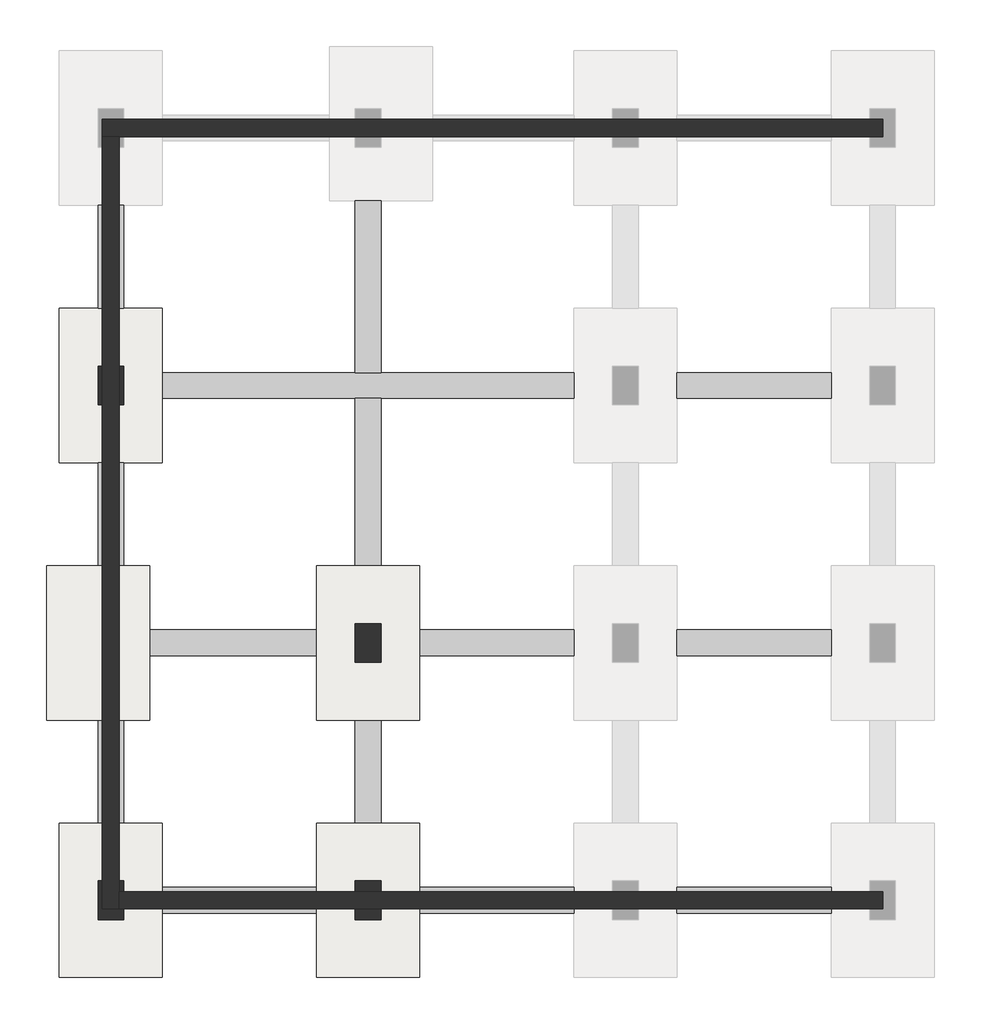
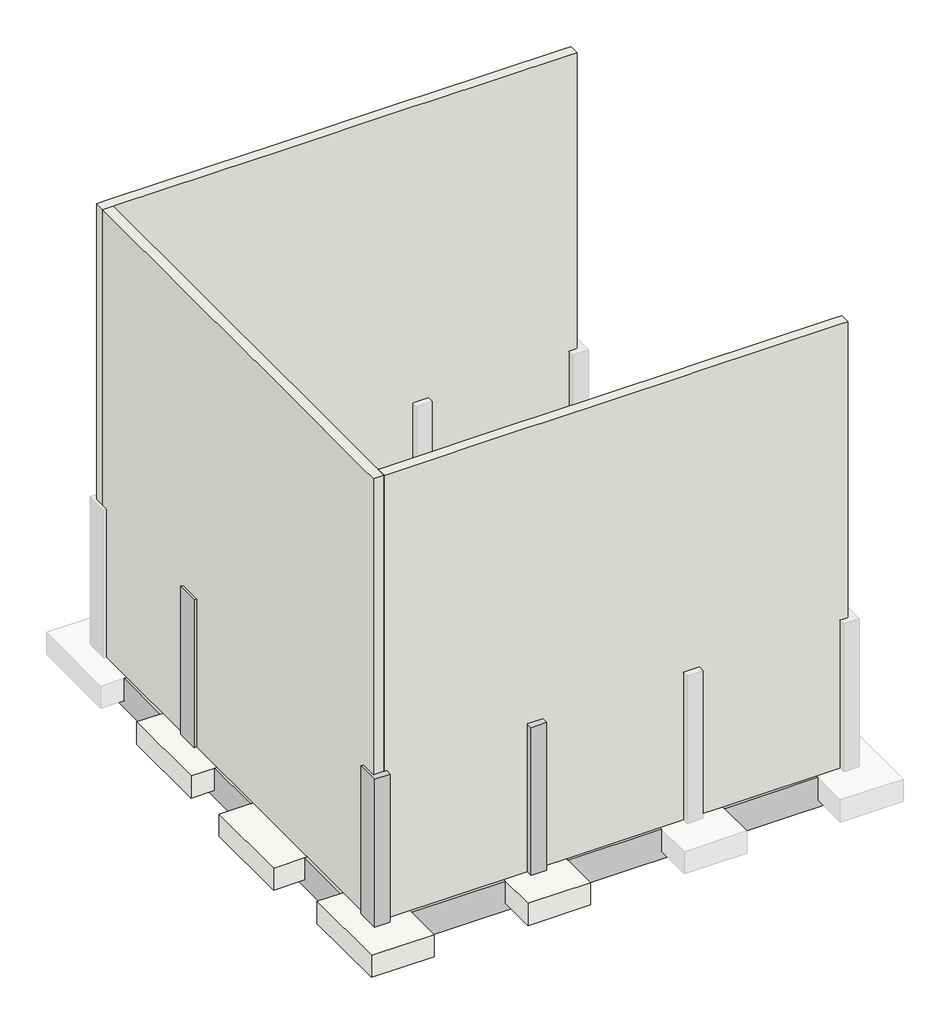
# One storey, part 1 of 2: 5 beams, 5 slabs, 4 columns, 3 walls.
"""IFC4 building model written with IfcOpenShell, lengths in millimetres."""

from ifc_helpers import new_model, si_unit, frame, origin, origin_with_axes, place, context, project, spatial, polyline, outline, extrude, faceted_brep, element, save

model = new_model("IFC4")

# Units and contexts
model_context = context("Model", 3, world=origin())
ifc_project = project(units=[si_unit("LENGTHUNIT", "METRE", prefix="MILLI")], contexts=[model_context])

# Site, building, storey
site = spatial("IfcSite", under=ifc_project)
building = spatial("IfcBuilding", under=site)
storey = spatial("IfcBuildingStorey", under=building, Elevation=0.0)

# Beams
placement = place(None, origin())
element("IfcBeam", 1, ObjectType="Concrete-Rectangular Beam : 12 x 24", at=placement, inside=storey, context=model_context, shape_type="Brep", body=[
    faceted_brep([(-21232.5609662, 3631.9972109, 0.0), (-21232.5609662, 3327.1972109, 0.0), (-19403.7609662, 3327.1972109, 0.0), (-19403.7609662, 3631.9972109, 0.0), (-21994.5609662, 3631.9972109, -457.2), (-21689.7609662, 3631.9972109, -457.2), (-21232.5609662, 3631.9972109, -457.2), (-19403.7609662, 3631.9972109, -457.2), (-18946.5609662, 3631.9972109, -457.2), (-18641.7609662, 3631.9972109, -457.2), (-18184.5609662, 3631.9972109, -457.2), (-18184.5609662, 3631.9972109, 0.0), (-16355.7609662, 3631.9972109, 0.0), (-16355.7609662, 3631.9972109, -457.2), (-15898.5609662, 3631.9972109, -457.2), (-15593.7609662, 3631.9972109, -457.2), (-15136.5609662, 3631.9972109, -457.2), (-15136.5609662, 3631.9972109, 0.0), (-13307.7609662, 3631.9972109, 0.0), (-13307.7609662, 3631.9972109, -457.2), (-12850.5609662, 3631.9972109, -457.2), (-12850.5609662, 3631.9972109, -609.6), (-15593.7609662, 3631.9972109, -609.6), (-15898.5609662, 3631.9972109, -609.6), (-18641.7609662, 3631.9972109, -609.6), (-18946.5609662, 3631.9972109, -609.6), (-21689.7609662, 3631.9972109, -609.6), (-21994.5609662, 3631.9972109, -609.6), (-12850.5609662, 3377.9972109, -609.6), (-12698.1609662, 3377.9972109, -609.6), (-12698.1609662, 3327.1972109, -609.6), (-21994.5609662, 3327.1972109, -609.6), (-21232.5609662, 3327.1972109, -457.2), (-21994.5609662, 3327.1972109, -457.2), (-12698.1609662, 3327.1972109, -457.2), (-13307.7609662, 3327.1972109, -457.2), (-13307.7609662, 3327.1972109, 0.0), (-15136.5609662, 3327.1972109, 0.0), (-15136.5609662, 3327.1972109, -457.2), (-16355.7609662, 3327.1972109, -457.2), (-16355.7609662, 3327.1972109, 0.0), (-18184.5609662, 3327.1972109, 0.0), (-18184.5609662, 3327.1972109, -457.2), (-19403.7609662, 3327.1972109, -457.2), (-12850.5609662, 3377.9972109, -457.2), (-12698.1609662, 3377.9972109, -457.2)], [[[0, 1, 2, 3]], [[4, 5, 6, 0, 3, 7, 8, 9, 10, 11, 12, 13, 14, 15, 16, 17, 18, 19, 20, 21, 22, 23, 24, 25, 26, 27]], [[21, 28, 29, 30, 31, 27, 26, 25, 24, 23, 22]], [[32, 33, 31, 30, 34, 35, 36, 37, 38, 39, 40, 41, 42, 43, 2, 1]], [[28, 21, 20, 44]], [[32, 6, 5, 4, 33]], [[6, 32, 1, 0]], [[42, 10, 9, 8, 7, 43]], [[10, 42, 41, 11]], [[43, 7, 3, 2]], [[11, 41, 40, 12]], [[38, 16, 15, 14, 13, 39]], [[16, 38, 37, 17]], [[39, 13, 12, 40]], [[17, 37, 36, 18]], [[19, 35, 34, 45, 44, 20]], [[35, 19, 18, 36]], [[27, 31, 33, 4]], [[30, 29, 45, 34]], [[29, 28, 44, 45]]]),
])
element("IfcBeam", 2, ObjectType="Concrete-Rectangular Beam : 12 x 24", at=placement, inside=storey, context=model_context, shape_type="Brep", body=[
    faceted_brep([(-21689.7609662, 11709.1972109, 0.0), (-21994.5609662, 11709.1972109, 0.0), (-21994.5609662, 10489.9972109, 0.0), (-21689.7609662, 10489.9972109, 0.0), (-21689.7609662, 12471.1972109, -609.6), (-21689.7609662, 12471.1972109, -457.2), (-21689.7609662, 11709.1972109, -457.2), (-21689.7609662, 10489.9972109, -457.2), (-21689.7609662, 9727.9972109, -457.2), (-21689.7609662, 9423.1972109, -457.2), (-21689.7609662, 8661.1972109, -457.2), (-21689.7609662, 8661.1972109, 0.0), (-21689.7609662, 7441.9972109, 0.0), (-21689.7609662, 7441.9972109, -457.2), (-21689.7609662, 6679.9972109, -457.2), (-21689.7609662, 6375.1972109, -457.2), (-21689.7609662, 5613.1972109, -457.2), (-21689.7609662, 5613.1972109, 0.0), (-21689.7609662, 4393.9972109, 0.0), (-21689.7609662, 4393.9972109, -457.2), (-21689.7609662, 3631.9972109, -457.2), (-21689.7609662, 3631.9972109, -609.6), (-21689.7609662, 6375.1972109, -609.6), (-21689.7609662, 6679.9972109, -609.6), (-21689.7609662, 9423.1972109, -609.6), (-21689.7609662, 9727.9972109, -609.6), (-21994.5609662, 12471.1972109, -609.6), (-21994.5609662, 3631.9972109, -609.6), (-21994.5609662, 12471.1972109, -457.2), (-21994.5609662, 3631.9972109, -457.2), (-21994.5609662, 4393.9972109, -457.2), (-21994.5609662, 4393.9972109, 0.0), (-21994.5609662, 5613.1972109, 0.0), (-21994.5609662, 5613.1972109, -457.2), (-21994.5609662, 7441.9972109, -457.2), (-21994.5609662, 7441.9972109, 0.0), (-21994.5609662, 8661.1972109, 0.0), (-21994.5609662, 8661.1972109, -457.2), (-21994.5609662, 10489.9972109, -457.2), (-21994.5609662, 11709.1972109, -457.2)], [[[0, 1, 2, 3]], [[4, 5, 6, 0, 3, 7, 8, 9, 10, 11, 12, 13, 14, 15, 16, 17, 18, 19, 20, 21, 22, 23, 24, 25]], [[26, 4, 25, 24, 23, 22, 21, 27]], [[28, 26, 27, 29, 30, 31, 32, 33, 34, 35, 36, 37, 38, 2, 1, 39]], [[4, 26, 28, 5]], [[27, 21, 20, 29]], [[39, 6, 5, 28]], [[6, 39, 1, 0]], [[37, 10, 9, 8, 7, 38]], [[10, 37, 36, 11]], [[38, 7, 3, 2]], [[11, 36, 35, 12]], [[19, 30, 29, 20]], [[30, 19, 18, 31]], [[33, 16, 15, 14, 13, 34]], [[16, 33, 32, 17]], [[34, 13, 12, 35]], [[31, 18, 17, 32]]]),
])
element("IfcBeam", 3, ObjectType="Concrete-Rectangular Beam : 12 x 24", at=placement, inside=storey, context=model_context, shape_type="Brep", body=[
    faceted_brep([(-15136.5609662, 9727.9972109, 0.0), (-15136.5609662, 9423.1972109, 0.0), (-13307.7609662, 9423.1972109, 0.0), (-13307.7609662, 9727.9972109, 0.0), (-21689.7609662, 9423.1972109, -609.6), (-18946.5609662, 9423.1972109, -609.6), (-18641.7609662, 9423.1972109, -609.6), (-15898.5609662, 9423.1972109, -609.6), (-15593.7609662, 9423.1972109, -609.6), (-12850.5609662, 9423.1972109, -609.6), (-12850.5609662, 9423.1972109, -457.2), (-13307.7609662, 9423.1972109, -457.2), (-15136.5609662, 9423.1972109, -457.2), (-15593.7609662, 9423.1972109, -457.2), (-15898.5609662, 9423.1972109, -457.2), (-16355.7609662, 9423.1972109, -457.2), (-16355.7609662, 9423.1972109, 0.0), (-18641.7609662, 9423.1972109, 0.0), (-18946.5609662, 9423.1972109, 0.0), (-21232.5609662, 9423.1972109, 0.0), (-21232.5609662, 9423.1972109, -457.2), (-21689.7609662, 9423.1972109, -457.2), (-12850.5609662, 9727.9972109, -609.6), (-21689.7609662, 9727.9972109, -609.6), (-18946.5609662, 9727.9972109, -609.6), (-18641.7609662, 9727.9972109, -609.6), (-15898.5609662, 9727.9972109, -609.6), (-15593.7609662, 9727.9972109, -609.6), (-21689.7609662, 9727.9972109, -457.2), (-21232.5609662, 9727.9972109, -457.2), (-21232.5609662, 9727.9972109, 0.0), (-18946.5609662, 9727.9972109, 0.0), (-18641.7609662, 9727.9972109, 0.0), (-16355.7609662, 9727.9972109, 0.0), (-16355.7609662, 9727.9972109, -457.2), (-15898.5609662, 9727.9972109, -457.2), (-15593.7609662, 9727.9972109, -457.2), (-15136.5609662, 9727.9972109, -457.2), (-13307.7609662, 9727.9972109, -457.2), (-12850.5609662, 9727.9972109, -457.2)], [[[0, 1, 2, 3]], [[4, 5, 6, 7, 8, 9, 10, 11, 2, 1, 12, 13, 14, 15, 16, 17, 18, 19, 20, 21]], [[22, 9, 8, 7, 6, 5, 4, 23, 24, 25, 26, 27]], [[22, 27, 26, 25, 24, 23, 28, 29, 30, 31, 32, 33, 34, 35, 36, 37, 0, 3, 38, 39]], [[9, 22, 39, 10]], [[23, 4, 21, 28]], [[20, 29, 28, 21]], [[29, 20, 19, 30]], [[12, 37, 36, 35, 34, 15, 14, 13]], [[37, 12, 1, 0]], [[15, 34, 33, 16]], [[38, 11, 10, 39]], [[11, 38, 3, 2]], [[30, 19, 18, 17, 16, 33, 32, 31]]]),
])
element("IfcBeam", 4, ObjectType="Concrete-Rectangular Beam : 12 x 24", at=placement, inside=storey, context=model_context, shape_type="Brep", body=[
    faceted_brep([(-15136.5609662, 6679.9972109, 0.0), (-15136.5609662, 6375.1972109, 0.0), (-13307.7609662, 6375.1972109, 0.0), (-13307.7609662, 6679.9972109, 0.0), (-21689.7609662, 6375.1972109, -609.6), (-18946.5609662, 6375.1972109, -609.6), (-18641.7609662, 6375.1972109, -609.6), (-15898.5609662, 6375.1972109, -609.6), (-15593.7609662, 6375.1972109, -609.6), (-12850.5609662, 6375.1972109, -609.6), (-12850.5609662, 6375.1972109, -457.2), (-13307.7609662, 6375.1972109, -457.2), (-15136.5609662, 6375.1972109, -457.2), (-15593.7609662, 6375.1972109, -457.2), (-15898.5609662, 6375.1972109, -457.2), (-16355.7609662, 6375.1972109, -457.2), (-16355.7609662, 6375.1972109, 0.0), (-18184.5609662, 6375.1972109, 0.0), (-18184.5609662, 6375.1972109, -457.2), (-18641.7609662, 6375.1972109, -457.2), (-18946.5609662, 6375.1972109, -457.2), (-19403.7609662, 6375.1972109, -457.2), (-19403.7609662, 6375.1972109, 0.0), (-21384.9609662, 6375.1972109, 0.0), (-21384.9609662, 6375.1972109, -457.2), (-21689.7609662, 6375.1972109, -457.2), (-12850.5609662, 6679.9972109, -609.6), (-21689.7609662, 6679.9972109, -609.6), (-18946.5609662, 6679.9972109, -609.6), (-18641.7609662, 6679.9972109, -609.6), (-15898.5609662, 6679.9972109, -609.6), (-15593.7609662, 6679.9972109, -609.6), (-21689.7609662, 6679.9972109, -457.2), (-21384.9609662, 6679.9972109, -457.2), (-21384.9609662, 6679.9972109, 0.0), (-19403.7609662, 6679.9972109, 0.0), (-19403.7609662, 6679.9972109, -457.2), (-18946.5609662, 6679.9972109, -457.2), (-18641.7609662, 6679.9972109, -457.2), (-18184.5609662, 6679.9972109, -457.2), (-18184.5609662, 6679.9972109, 0.0), (-16355.7609662, 6679.9972109, 0.0), (-16355.7609662, 6679.9972109, -457.2), (-15898.5609662, 6679.9972109, -457.2), (-15593.7609662, 6679.9972109, -457.2), (-15136.5609662, 6679.9972109, -457.2), (-13307.7609662, 6679.9972109, -457.2), (-12850.5609662, 6679.9972109, -457.2)], [[[0, 1, 2, 3]], [[4, 5, 6, 7, 8, 9, 10, 11, 2, 1, 12, 13, 14, 15, 16, 17, 18, 19, 20, 21, 22, 23, 24, 25]], [[26, 9, 8, 7, 6, 5, 4, 27, 28, 29, 30, 31]], [[26, 31, 30, 29, 28, 27, 32, 33, 34, 35, 36, 37, 38, 39, 40, 41, 42, 43, 44, 45, 0, 3, 46, 47]], [[9, 26, 47, 10]], [[27, 4, 25, 32]], [[18, 39, 38, 37, 36, 21, 20, 19]], [[39, 18, 17, 40]], [[21, 36, 35, 22]], [[22, 35, 34, 23]], [[12, 45, 44, 43, 42, 15, 14, 13]], [[45, 12, 1, 0]], [[15, 42, 41, 16]], [[40, 17, 16, 41]], [[46, 11, 10, 47]], [[11, 46, 3, 2]], [[24, 33, 32, 25]], [[33, 24, 23, 34]]]),
])
element("IfcBeam", 5, ObjectType="Concrete-Rectangular Beam : 12 x 24", at=placement, inside=storey, context=model_context, shape_type="SweptSolid", body=[
    extrude(outline(polyline([(5613.1972109, 0.0), (5613.1972109, -457.2), (6375.1972109, -457.2), (6375.1972109, -609.6), (3631.9972109, -609.6), (3631.9972109, -457.2), (4393.9972109, -457.2), (4393.9972109, 0.0), (5613.1972109, 0.0)])), frame((-18946.5609662, 0.0, 0.0), z_axis=(1.0, 0.0, 0.0), x_axis=(0.0, 1.0, 0.0)), (0.0, 0.0, 1.0), 304.8),
    extrude(outline(polyline([(12471.1972109, -609.6), (9727.9972109, -609.6), (9727.9972109, 0.0), (11759.9972109, 0.0), (11759.9972109, -457.2), (12471.1972109, -457.2), (12471.1972109, -609.6)])), frame((-18946.5609662, 0.0, 0.0), z_axis=(1.0, 0.0, 0.0), x_axis=(0.0, 1.0, 0.0)), (0.0, 0.0, 1.0), 304.8),
    extrude(outline(polyline([(7441.9972109, -457.2), (7441.9972109, 0.0), (9423.1972109, 0.0), (9423.1972109, -609.6), (6679.9972109, -609.6), (6679.9972109, -457.2), (7441.9972109, -457.2)])), frame((-18946.5609662, 0.0, 0.0), z_axis=(1.0, 0.0, 0.0), x_axis=(0.0, 1.0, 0.0)), (0.0, 0.0, 1.0), 304.8),
])

# Columns
element("IfcColumn", 6, ObjectType="Concrete-Rectangular-Column : 12 x 18", at=placement, inside=storey, context=model_context, shape_type="Brep", body=[
    faceted_brep([(-21689.7609662, 9804.1972109, 0.0), (-21689.7609662, 9346.9972109, 0.0), (-21740.5609662, 9346.9972109, 0.0), (-21740.5609662, 9804.1972109, 0.0), (-21689.7609662, 9804.1972109, 3048.0), (-21689.7609662, 9804.1972109, 2895.6), (-21689.7609662, 9804.1972109, 2438.4), (-21740.5609662, 9804.1972109, 2438.4), (-21740.5609662, 9804.1972109, 2895.6), (-21740.5609662, 9804.1972109, 3048.0), (-21689.7609662, 9346.9972109, 3048.0), (-21689.7609662, 9346.9972109, 2895.6), (-21689.7609662, 9346.9972109, 2438.4), (-21740.5609662, 9346.9972109, 3048.0), (-21740.5609662, 9346.9972109, 2895.6), (-21740.5609662, 9346.9972109, 2438.4)], [[[0, 1, 2, 3]], [[4, 5, 6, 0, 3, 7, 8, 9]], [[1, 0, 6, 5, 4, 10, 11, 12]], [[1, 12, 11, 10, 13, 14, 15, 2]], [[3, 2, 15, 14, 13, 9, 8, 7]], [[10, 4, 9, 13]]]),
    faceted_brep([(-21994.5609662, 9804.1972109, 0.0), (-21994.5609662, 9346.9972109, 0.0), (-21994.5609662, 9346.9972109, 2438.4), (-21994.5609662, 9346.9972109, 3048.0), (-21994.5609662, 9804.1972109, 3048.0), (-21994.5609662, 9804.1972109, 2438.4), (-21943.7609662, 9346.9972109, 3048.0), (-21943.7609662, 9804.1972109, 3048.0), (-21943.7609662, 9346.9972109, 0.0), (-21943.7609662, 9804.1972109, 0.0), (-21943.7609662, 9804.1972109, 2438.4), (-21943.7609662, 9346.9972109, 2438.4)], [[[0, 1, 2, 3, 4, 5]], [[4, 3, 6, 7]], [[8, 9, 10, 7, 6, 11]], [[1, 0, 9, 8]], [[0, 5, 4, 7, 10, 9]], [[3, 2, 1, 8, 11, 6]]]),
])
element("IfcColumn", 7, ObjectType="Concrete-Rectangular-Column : 12 x 18", at=placement, inside=storey, context=model_context, shape_type="Brep", body=[
    faceted_brep([(-21740.5609662, 3708.1972109, 0.0), (-21689.7609662, 3708.1972109, 0.0), (-21689.7609662, 3581.1972109, 0.0), (-21740.5609662, 3581.1972109, 0.0), (-21689.7609662, 3708.1972109, 3048.0), (-21740.5609662, 3708.1972109, 3048.0), (-21740.5609662, 3581.1972109, 3048.0), (-21689.7609662, 3581.1972109, 3048.0)], [[[0, 1, 2, 3]], [[4, 1, 0, 5]], [[5, 0, 3, 6]], [[3, 2, 7, 6]], [[1, 4, 7, 2]], [[4, 5, 6, 7]]]),
    faceted_brep([(-21994.5609662, 3708.1972109, 0.0), (-21994.5609662, 3250.9972109, 0.0), (-21994.5609662, 3250.9972109, 3048.0), (-21994.5609662, 3708.1972109, 3048.0), (-21689.7609662, 3250.9972109, 3048.0), (-21689.7609662, 3250.9972109, 0.0), (-21689.7609662, 3377.9972109, 0.0), (-21689.7609662, 3377.9972109, 3048.0), (-21943.7609662, 3377.9972109, 3048.0), (-21943.7609662, 3708.1972109, 3048.0), (-21943.7609662, 3377.9972109, 0.0), (-21943.7609662, 3708.1972109, 0.0), (-21740.5609662, 3377.9972109, 0.0)], [[[0, 1, 2, 3]], [[4, 5, 6, 7]], [[1, 5, 4, 2]], [[3, 2, 4, 7, 8, 9]], [[10, 11, 9, 8]], [[0, 3, 9, 11]], [[10, 8, 7, 6, 12]], [[1, 0, 11, 10, 12, 6, 5]]]),
])
element("IfcColumn", 8, ObjectType="Concrete-Rectangular-Column : 12 x 18", at=placement, inside=storey, context=model_context, shape_type="SweptSolid", body=[
    extrude(outline(polyline([(-18946.5609662, 6298.9972109), (-18946.5609662, 6756.1972109), (-18641.7609662, 6756.1972109), (-18641.7609662, 6298.9972109), (-18946.5609662, 6298.9972109)])), origin_with_axes(), (0.0, 0.0, 1.0), 3048.0),
])
element("IfcColumn", 9, ObjectType="Concrete-Rectangular-Column : 12 x 18", at=placement, inside=storey, context=model_context, shape_type="Brep", body=[
    faceted_brep([(-18641.7609662, 3250.9972109, 0.0), (-18946.5609662, 3250.9972109, 0.0), (-18946.5609662, 3377.9972109, 0.0), (-18641.7609662, 3377.9972109, 0.0), (-18641.7609662, 3250.9972109, 3048.0), (-18641.7609662, 3377.9972109, 2438.4), (-18641.7609662, 3377.9972109, 3048.0), (-18641.7609662, 3327.1972109, 3048.0), (-18946.5609662, 3250.9972109, 3048.0), (-18946.5609662, 3377.9972109, 2438.4), (-18946.5609662, 3377.9972109, 3048.0), (-18946.5609662, 3327.1972109, 3048.0)], [[[0, 1, 2, 3]], [[4, 0, 3, 5, 6, 7]], [[1, 0, 4, 8]], [[3, 2, 9, 10, 6, 5]], [[1, 8, 11, 10, 9, 2]], [[8, 4, 7, 6, 10, 11]]]),
    faceted_brep([(-18946.5609662, 3708.1972109, 3048.0), (-18946.5609662, 3708.1972109, 0.0), (-18946.5609662, 3581.1972109, 0.0), (-18946.5609662, 3581.1972109, 2438.4), (-18946.5609662, 3581.1972109, 2895.6), (-18946.5609662, 3581.1972109, 3048.0), (-18641.7609662, 3708.1972109, 0.0), (-18641.7609662, 3708.1972109, 3048.0), (-18641.7609662, 3581.1972109, 3048.0), (-18641.7609662, 3581.1972109, 0.0), (-18641.7609662, 3581.1972109, 2438.4), (-18641.7609662, 3581.1972109, 2895.6)], [[[0, 1, 2, 3, 4, 5]], [[6, 1, 0, 7]], [[7, 0, 5, 8]], [[2, 9, 10, 11, 8, 5, 4, 3]], [[1, 6, 9, 2]], [[6, 7, 8, 11, 10, 9]]]),
])

# Slabs
element("IfcSlab", 10, ObjectType="Footing-Rectangular : 72\" x 48\" x 18\"", at=placement, inside=storey, context=model_context, shape_type="Brep", body=[
    faceted_brep([(-22451.7609662, 8661.1972109, 0.0), (-21994.5609662, 8661.1972109, 0.0), (-21689.7609662, 8661.1972109, 0.0), (-21232.5609662, 8661.1972109, 0.0), (-21232.5609662, 9423.1972109, 0.0), (-21232.5609662, 9727.9972109, 0.0), (-21232.5609662, 10489.9972109, 0.0), (-21689.7609662, 10489.9972109, 0.0), (-21994.5609662, 10489.9972109, 0.0), (-22451.7609662, 10489.9972109, 0.0), (-22451.7609662, 8661.1972109, -457.2), (-22451.7609662, 10489.9972109, -457.2), (-21994.5609662, 10489.9972109, -457.2), (-21689.7609662, 10489.9972109, -457.2), (-21232.5609662, 10489.9972109, -457.2), (-21232.5609662, 9727.9972109, -457.2), (-21232.5609662, 9423.1972109, -457.2), (-21232.5609662, 8661.1972109, -457.2), (-21689.7609662, 8661.1972109, -457.2), (-21994.5609662, 8661.1972109, -457.2)], [[[0, 1, 2, 3, 4, 5, 6, 7, 8, 9]], [[10, 11, 12, 13, 14, 15, 16, 17, 18, 19]], [[3, 2, 1, 0, 10, 19, 18, 17]], [[6, 5, 4, 3, 17, 16, 15, 14]], [[9, 8, 7, 6, 14, 13, 12, 11]], [[0, 9, 11, 10]]]),
])
element("IfcSlab", 11, ObjectType="Footing-Rectangular : 72\" x 48\" x 18\"", at=placement, inside=storey, context=model_context, shape_type="Brep", body=[
    faceted_brep([(-22451.7609662, 2565.1972109, 0.0), (-21232.5609662, 2565.1972109, 0.0), (-21232.5609662, 3327.1972109, 0.0), (-21232.5609662, 3631.9972109, 0.0), (-21232.5609662, 4393.9972109, 0.0), (-21689.7609662, 4393.9972109, 0.0), (-21994.5609662, 4393.9972109, 0.0), (-22451.7609662, 4393.9972109, 0.0), (-22451.7609662, 2565.1972109, -457.2), (-22451.7609662, 4393.9972109, -457.2), (-21994.5609662, 4393.9972109, -457.2), (-21689.7609662, 4393.9972109, -457.2), (-21232.5609662, 4393.9972109, -457.2), (-21232.5609662, 3631.9972109, -457.2), (-21232.5609662, 3327.1972109, -457.2), (-21232.5609662, 2565.1972109, -457.2)], [[[0, 1, 2, 3, 4, 5, 6, 7]], [[8, 9, 10, 11, 12, 13, 14, 15]], [[1, 0, 8, 15]], [[4, 3, 2, 1, 15, 14, 13, 12]], [[7, 6, 5, 4, 12, 11, 10, 9]], [[0, 7, 9, 8]]]),
])
element("IfcSlab", 12, ObjectType="Footing-Rectangular : 72\" x 48\" x 18\"", at=placement, inside=storey, context=model_context, shape_type="Brep", body=[
    faceted_brep([(-19403.7609662, 5613.1972109, 0.0), (-18946.5609662, 5613.1972109, 0.0), (-18641.7609662, 5613.1972109, 0.0), (-18184.5609662, 5613.1972109, 0.0), (-18184.5609662, 6375.1972109, 0.0), (-18184.5609662, 6679.9972109, 0.0), (-18184.5609662, 7441.9972109, 0.0), (-18641.7609662, 7441.9972109, 0.0), (-18946.5609662, 7441.9972109, 0.0), (-19403.7609662, 7441.9972109, 0.0), (-19403.7609662, 6679.9972109, 0.0), (-19403.7609662, 6375.1972109, 0.0), (-19403.7609662, 5613.1972109, -457.2), (-19403.7609662, 6375.1972109, -457.2), (-19403.7609662, 6679.9972109, -457.2), (-19403.7609662, 7441.9972109, -457.2), (-18946.5609662, 7441.9972109, -457.2), (-18641.7609662, 7441.9972109, -457.2), (-18184.5609662, 7441.9972109, -457.2), (-18184.5609662, 6679.9972109, -457.2), (-18184.5609662, 6375.1972109, -457.2), (-18184.5609662, 5613.1972109, -457.2), (-18641.7609662, 5613.1972109, -457.2), (-18946.5609662, 5613.1972109, -457.2)], [[[0, 1, 2, 3, 4, 5, 6, 7, 8, 9, 10, 11]], [[12, 13, 14, 15, 16, 17, 18, 19, 20, 21, 22, 23]], [[3, 2, 1, 0, 12, 23, 22, 21]], [[6, 5, 4, 3, 21, 20, 19, 18]], [[9, 8, 7, 6, 18, 17, 16, 15]], [[0, 11, 10, 9, 15, 14, 13, 12]]]),
])
element("IfcSlab", 13, ObjectType="Footing-Rectangular : 72\" x 48\" x 18\"", at=placement, inside=storey, context=model_context, shape_type="Brep", body=[
    faceted_brep([(-19403.7609662, 2565.1972109, 0.0), (-18184.5609662, 2565.1972109, 0.0), (-18184.5609662, 3327.1972109, 0.0), (-18184.5609662, 3631.9972109, 0.0), (-18184.5609662, 4393.9972109, 0.0), (-18641.7609662, 4393.9972109, 0.0), (-18946.5609662, 4393.9972109, 0.0), (-19403.7609662, 4393.9972109, 0.0), (-19403.7609662, 3631.9972109, 0.0), (-19403.7609662, 3327.1972109, 0.0), (-19403.7609662, 2565.1972109, -457.2), (-19403.7609662, 3327.1972109, -457.2), (-19403.7609662, 3631.9972109, -457.2), (-19403.7609662, 4393.9972109, -457.2), (-18946.5609662, 4393.9972109, -457.2), (-18641.7609662, 4393.9972109, -457.2), (-18184.5609662, 4393.9972109, -457.2), (-18184.5609662, 3631.9972109, -457.2), (-18184.5609662, 3327.1972109, -457.2), (-18184.5609662, 2565.1972109, -457.2)], [[[0, 1, 2, 3, 4, 5, 6, 7, 8, 9]], [[10, 11, 12, 13, 14, 15, 16, 17, 18, 19]], [[1, 0, 10, 19]], [[4, 3, 2, 1, 19, 18, 17, 16]], [[7, 6, 5, 4, 16, 15, 14, 13]], [[0, 9, 8, 7, 13, 12, 11, 10]]]),
])
element("IfcSlab", 14, ObjectType="Footing-Rectangular : 72\" x 48\" x 18\"", at=placement, inside=storey, context=model_context, shape_type="Brep", body=[
    faceted_brep([(-22604.1609662, 5613.1972109, 0.0), (-21994.5609662, 5613.1972109, 0.0), (-21689.7609662, 5613.1972109, 0.0), (-21384.9609662, 5613.1972109, 0.0), (-21384.9609662, 6375.1972109, 0.0), (-21384.9609662, 6679.9972109, 0.0), (-21384.9609662, 7441.9972109, 0.0), (-21689.7609662, 7441.9972109, 0.0), (-21994.5609662, 7441.9972109, 0.0), (-22604.1609662, 7441.9972109, 0.0), (-22604.1609662, 5613.1972109, -457.2), (-22604.1609662, 7441.9972109, -457.2), (-21994.5609662, 7441.9972109, -457.2), (-21689.7609662, 7441.9972109, -457.2), (-21384.9609662, 7441.9972109, -457.2), (-21384.9609662, 6679.9972109, -457.2), (-21384.9609662, 6375.1972109, -457.2), (-21384.9609662, 5613.1972109, -457.2), (-21689.7609662, 5613.1972109, -457.2), (-21994.5609662, 5613.1972109, -457.2)], [[[0, 1, 2, 3, 4, 5, 6, 7, 8, 9]], [[10, 11, 12, 13, 14, 15, 16, 17, 18, 19]], [[3, 2, 1, 0, 10, 19, 18, 17]], [[6, 5, 4, 3, 17, 16, 15, 14]], [[9, 8, 7, 6, 14, 13, 12, 11]], [[0, 9, 11, 10]]]),
])

# Walls
element("IfcWall", 15, ObjectType="Generic - 8\"", at=placement, inside=storey, context=model_context, shape_type="Brep", body=[
    faceted_brep([(-21943.7609662, 12521.9972109, 0.0), (-21740.5609662, 12521.9972109, 0.0), (-21689.7609662, 12521.9972109, 0.0), (-18946.5609662, 12521.9972109, 0.0), (-18641.7609662, 12521.9972109, 0.0), (-15898.5609662, 12521.9972109, 0.0), (-15593.7609662, 12521.9972109, 0.0), (-12850.5609662, 12521.9972109, 0.0), (-12698.1609662, 12521.9972109, 0.0), (-12698.1609662, 12521.9972109, 3048.0), (-12698.1609662, 12521.9972109, 6096.0), (-12698.1609662, 12521.9972109, 9144.0), (-12850.5609662, 12521.9972109, 9144.0), (-15593.7609662, 12521.9972109, 9144.0), (-15898.5609662, 12521.9972109, 9144.0), (-18641.7609662, 12521.9972109, 9144.0), (-18946.5609662, 12521.9972109, 9144.0), (-21689.7609662, 12521.9972109, 9144.0), (-21740.5609662, 12521.9972109, 9144.0), (-21943.7609662, 12521.9972109, 9144.0), (-21943.7609662, 12725.1972109, 0.0), (-21943.7609662, 12725.1972109, 3048.0), (-21943.7609662, 12725.1972109, 6096.0), (-21943.7609662, 12725.1972109, 9144.0), (-21689.7609662, 12725.1972109, 9144.0), (-18946.5609662, 12725.1972109, 9144.0), (-18641.7609662, 12725.1972109, 9144.0), (-15898.5609662, 12725.1972109, 9144.0), (-15593.7609662, 12725.1972109, 9144.0), (-12850.5609662, 12725.1972109, 9144.0), (-12698.1609662, 12725.1972109, 9144.0), (-12698.1609662, 12725.1972109, 6096.0), (-12698.1609662, 12725.1972109, 3048.0), (-12698.1609662, 12725.1972109, 0.0), (-12850.5609662, 12725.1972109, 0.0), (-15593.7609662, 12725.1972109, 0.0), (-15898.5609662, 12725.1972109, 0.0), (-18641.7609662, 12725.1972109, 0.0), (-18946.5609662, 12725.1972109, 0.0), (-21689.7609662, 12725.1972109, 0.0)], [[[0, 1, 2, 3, 4, 5, 6, 7, 8, 9, 10, 11, 12, 13, 14, 15, 16, 17, 18, 19]], [[20, 21, 22, 23, 24, 25, 26, 27, 28, 29, 30, 31, 32, 33, 34, 35, 36, 37, 38, 39]], [[8, 7, 6, 5, 4, 3, 2, 1, 0, 20, 39, 38, 37, 36, 35, 34, 33]], [[11, 10, 9, 8, 33, 32, 31, 30]], [[19, 18, 17, 16, 15, 14, 13, 12, 11, 30, 29, 28, 27, 26, 25, 24, 23]], [[0, 19, 23, 22, 21, 20]]]),
])
element("IfcWall", 16, ObjectType="Generic - 8\"", at=placement, inside=storey, context=model_context, shape_type="Brep", body=[
    faceted_brep([(-21943.7609662, 12521.9972109, 0.0), (-21943.7609662, 12394.9972109, 0.0), (-21943.7609662, 9804.1972109, 0.0), (-21943.7609662, 9346.9972109, 0.0), (-21943.7609662, 3708.1972109, 0.0), (-21943.7609662, 3377.9972109, 0.0), (-21943.7609662, 3377.9972109, 3048.0), (-21943.7609662, 3377.9972109, 6096.0), (-21943.7609662, 3377.9972109, 9144.0), (-21943.7609662, 3708.1972109, 9144.0), (-21943.7609662, 6298.9972109, 9144.0), (-21943.7609662, 6756.1972109, 9144.0), (-21943.7609662, 9346.9972109, 9144.0), (-21943.7609662, 9804.1972109, 9144.0), (-21943.7609662, 12394.9972109, 9144.0), (-21943.7609662, 12521.9972109, 9144.0), (-21740.5609662, 12521.9972109, 0.0), (-21740.5609662, 12521.9972109, 3048.0), (-21740.5609662, 12521.9972109, 6096.0), (-21740.5609662, 12521.9972109, 9144.0), (-21740.5609662, 12394.9972109, 9144.0), (-21740.5609662, 9804.1972109, 9144.0), (-21740.5609662, 9346.9972109, 9144.0), (-21740.5609662, 6756.1972109, 9144.0), (-21740.5609662, 6298.9972109, 9144.0), (-21740.5609662, 3708.1972109, 9144.0), (-21740.5609662, 3581.1972109, 9144.0), (-21740.5609662, 3377.9972109, 9144.0), (-21740.5609662, 3377.9972109, 0.0), (-21740.5609662, 3581.1972109, 0.0), (-21740.5609662, 3708.1972109, 0.0), (-21740.5609662, 9346.9972109, 0.0), (-21740.5609662, 9804.1972109, 0.0), (-21740.5609662, 12394.9972109, 0.0)], [[[0, 1, 2, 3, 4, 5, 6, 7, 8, 9, 10, 11, 12, 13, 14, 15]], [[16, 17, 18, 19, 20, 21, 22, 23, 24, 25, 26, 27, 28, 29, 30, 31, 32, 33]], [[5, 4, 3, 2, 1, 0, 16, 33, 32, 31, 30, 29, 28]], [[15, 14, 13, 12, 11, 10, 9, 8, 27, 26, 25, 24, 23, 22, 21, 20, 19]], [[0, 15, 19, 18, 17, 16]], [[8, 7, 6, 5, 28, 27]]]),
])
element("IfcWall", 17, ObjectType="Generic - 8\"", at=placement, inside=storey, context=model_context, shape_type="Brep", body=[
    faceted_brep([(-21740.5609662, 3377.9972109, 0.0), (-21689.7609662, 3377.9972109, 0.0), (-18946.5609662, 3377.9972109, 0.0), (-18641.7609662, 3377.9972109, 0.0), (-15898.5609662, 3377.9972109, 0.0), (-15593.7609662, 3377.9972109, 0.0), (-12850.5609662, 3377.9972109, 0.0), (-12698.1609662, 3377.9972109, 0.0), (-12698.1609662, 3377.9972109, 3048.0), (-12698.1609662, 3377.9972109, 6096.0), (-12698.1609662, 3377.9972109, 9144.0), (-12850.5609662, 3377.9972109, 9144.0), (-15593.7609662, 3377.9972109, 9144.0), (-15898.5609662, 3377.9972109, 9144.0), (-18641.7609662, 3377.9972109, 9144.0), (-18946.5609662, 3377.9972109, 9144.0), (-21689.7609662, 3377.9972109, 9144.0), (-21740.5609662, 3377.9972109, 9144.0), (-21740.5609662, 3581.1972109, 0.0), (-21740.5609662, 3581.1972109, 3048.0), (-21740.5609662, 3581.1972109, 6096.0), (-21740.5609662, 3581.1972109, 9144.0), (-21689.7609662, 3581.1972109, 9144.0), (-18946.5609662, 3581.1972109, 9144.0), (-18641.7609662, 3581.1972109, 9144.0), (-15898.5609662, 3581.1972109, 9144.0), (-15593.7609662, 3581.1972109, 9144.0), (-12850.5609662, 3581.1972109, 9144.0), (-12698.1609662, 3581.1972109, 9144.0), (-12698.1609662, 3581.1972109, 6096.0), (-12698.1609662, 3581.1972109, 3048.0), (-12698.1609662, 3581.1972109, 0.0), (-12850.5609662, 3581.1972109, 0.0), (-15593.7609662, 3581.1972109, 0.0), (-15898.5609662, 3581.1972109, 0.0), (-18641.7609662, 3581.1972109, 0.0), (-18946.5609662, 3581.1972109, 0.0), (-21689.7609662, 3581.1972109, 0.0)], [[[0, 1, 2, 3, 4, 5, 6, 7, 8, 9, 10, 11, 12, 13, 14, 15, 16, 17]], [[18, 19, 20, 21, 22, 23, 24, 25, 26, 27, 28, 29, 30, 31, 32, 33, 34, 35, 36, 37]], [[7, 6, 5, 4, 3, 2, 1, 0, 18, 37, 36, 35, 34, 33, 32, 31]], [[10, 9, 8, 7, 31, 30, 29, 28]], [[17, 16, 15, 14, 13, 12, 11, 10, 28, 27, 26, 25, 24, 23, 22, 21]], [[0, 17, 21, 20, 19, 18]]]),
])

save(model, "model.ifc")

# Revit data of these elements
# Grids (mm)
#   "20": line (-12698.161, -7017.173) -> (-12698.161, 21483.293)
#   "5": line (-29159.894, 12623.597) -> (-7170.77, 12623.597)
#   "6": line (-29159.894, 9575.597) -> (-7170.77, 9575.597)
#   "7": line (-29159.894, 6527.597) -> (-7170.77, 6527.597)
#   "8": line (-29159.894, 3479.597) -> (-7170.77, 3479.597)
#   "1": line (-21842.161, -7017.173) -> (-21842.161, 21483.293)
#   "2": line (-18794.161, -7017.173) -> (-18794.161, 21483.293)
#   "4": line (-12698.161, -7017.173) -> (-12698.161, 21483.293)
#   "3": line (-15746.161, -7017.173) -> (-15746.161, 21483.293)
#   "9": line (-21842.161, -7017.173) -> (-21842.161, 21483.293)
#   "10": line (-18794.161, -7017.173) -> (-18794.161, 21483.293)
#   "11": line (-15746.161, -7017.173) -> (-15746.161, 21483.293)
#   "12": line (-12698.161, -7017.173) -> (-12698.161, 21483.293)
#   "18": line (-18794.161, -7017.173) -> (-18794.161, 21483.293)
#   "19": line (-15746.161, -7017.173) -> (-15746.161, 21483.293)
#   "17": line (-21842.161, -7017.173) -> (-21842.161, 21483.293)
# Type "Concrete-Rectangular Beam : 12 x 24"
#   Assembly Code = "B10"
#   Length [instance default] = 5' - 0"
#   b = 1' - 0"
#   h = 2' - 0"
#   Structural Material [instance default] = Concrete, Cast-in-Place gray
# Type "Concrete-Rectangular-Column : 12 x 18"
#   Assembly Code = "B10"
#   b = 1' - 0"
#   h = 1' - 6"
#   Structural Material [instance default] = Concrete, Cast-in-Place gray
# Type "Footing-Rectangular : 72\" x 48\" x 18\""
#   Assembly Code = "A1010100"
#   Width = 4' - 0"
#   Length = 6' - 0"
#   Foundation Thickness = 1' - 6"
#   Structural Material [instance default] = Concrete, Cast-in-Place gray
# Type "Generic - 8\""
#   Assembly Code = "B2010"
#   Layers, outside or top first: 0' - 8" no material (function 1)
# Elements 1, 2, 3, 4, 5 (IfcBeam, "Concrete-Rectangular Beam : 12 x 24")
#   Structural Material = Concrete, Cast-in-Place gray
#   Phase Created = New Construction
#   Materials on its faces: "Concrete, Cast-in-Place gray"
# Elements 6, 7, 8, 9 (IfcColumn, "Concrete-Rectangular-Column : 12 x 18")
#   Comments = ""
#   Structural Material = Concrete, Cast-in-Place gray
#   Phase Created = New Construction
#   Materials on its faces: "Concrete, Cast-in-Place gray"
# Elements 10, 11, 12, 13, 14 (IfcSlab, "Footing-Rectangular : 72\" x 48\" x 18\"")
#   Structural Material = Concrete, Cast-in-Place gray
#   Phase Created = New Construction
#   Materials on its faces: "Concrete, Cast-in-Place gray"
# Elements 15, 16, 17 (IfcWall, "Generic - 8\"")
#   Comments = ""
#   Top Offset = 0' - 0"
#   Base Offset = 0' - 0"
#   wall height = 30' - 0"
#   Phase Created = New Construction
#   Base Constraint = 00-GFL
#   Top Constraint = 03-TFL
#   Materials on its faces: "Default Wall"
# Materials
#   "Concrete, Cast-in-Place gray": class "Concrete", colour RGB 192 192 192, transparency 0, Description = "Cast-in-place concrete", Cost = 0
#   "Default Wall": colour RGB 128 128 128, transparency 0, Cost = 0
